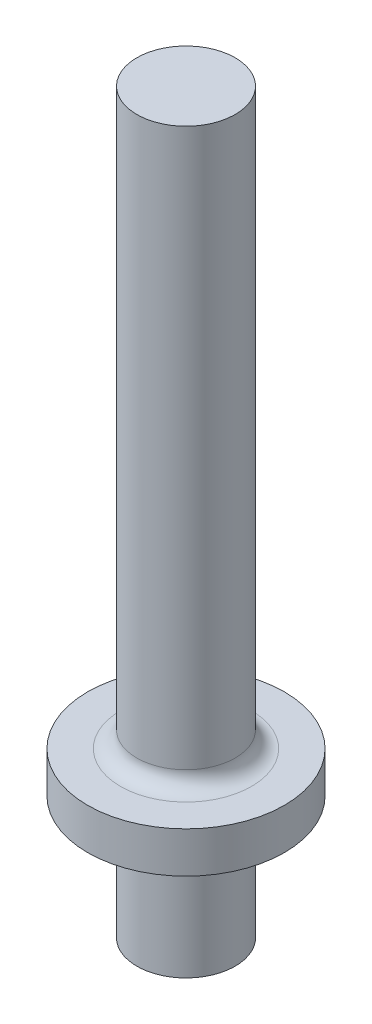
SolidWorks part; units mm, degrees
material "Plain Carbon Steel"
ref_plane "Front Plane" through (0, 0, 0) normal (0, 0, 1) x (1, 0, 0)
ref_plane "Top Plane" through (0, 0, 0) normal (0, 1, 0) x (1, 0, 0)
ref_plane "Right Plane" through (0, 0, 0) normal (1, 0, 0) x (0, 0, -1)
sketch "Stud Profile Sketch" plane through (0, 0, 0) normal (0, 0, 1) x (1, 0, 0)
  line L0 (0, -19.6575) -> (0, 124.5815) construction
  line L1 (0, 0) -> (6, 0)
  line L2 (6, 0) -> (6, 15)
  line L3 (6, 15) -> (12, 15)
  line L4 (12, 15) -> (12, 20)
  line L5 (12, 20) -> (6, 20)
  line L6 (6, 20) -> (6, 90)
  line L7 (6, 90) -> (0, 90)
  line L8 (0, 90) -> (0, 0)
  dimension "D1" = 6
  dimension "D2" = 12
  dimension "D3" = 5
  dimension "D4" = 15
  dimension "D5" = 90
revolve "Stud Body Revolve" add sketch "Stud Profile Sketch" angle 360 about L0
fillet "Collar Fillet R2" radius 2 1 edges at (0, 20, -6)
